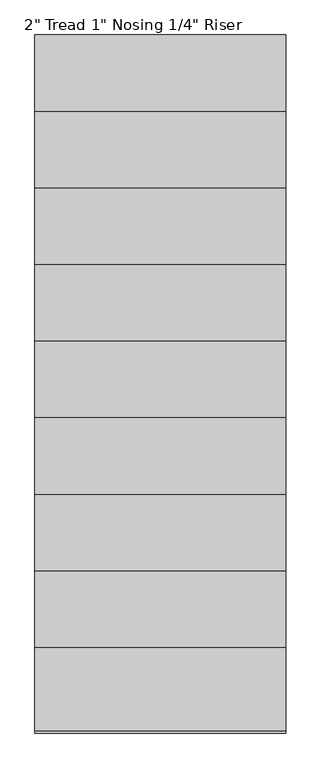
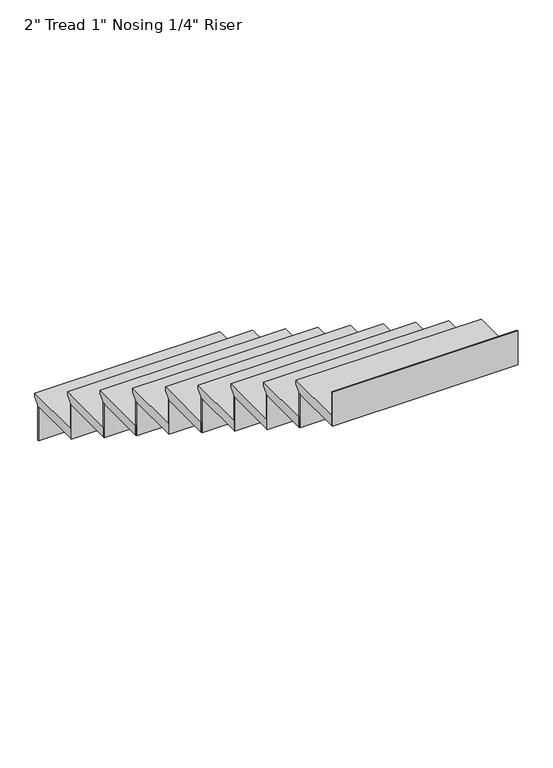
"""IFC4 building model written with IfcOpenShell, lengths in millimetres: stair flight geometry."""

from ifc_helpers import new_model, si_unit, frame, origin, place, context, project, spatial, polyline, outline, extrude, source, transform, mapped, element, save


def stair_flight_364c9dde(model_context):
    return source(origin(), model_context, "Body", "SweptSolid", [
        extrude(outline(polyline([(1808.6257925, 8610.6), (2113.4257925, 8610.6), (2113.4257925, 8591.55), (2088.0257925, 8566.15), (2088.0257925, 8559.8), (1808.6257925, 8559.8), (1808.6257925, 8610.6)])), frame((1465.4501403, 0.0, 0.0), z_axis=(1.0, 0.0, 0.0), x_axis=(0.0, 1.0, 0.0)), (0.0, 0.0, 1.0), 914.4),
        extrude(outline(polyline([(1465.4501403, 2081.6757925), (1465.4501403, 2088.0257925), (2379.8501403, 2088.0257925), (2379.8501403, 2081.6757925), (1465.4501403, 2081.6757925)])), frame((0.0, 0.0, 8382.0), z_axis=(0.0, 0.0, 1.0), x_axis=(1.0, 0.0, 0.0)), (0.0, 0.0, 1.0), 177.8),
        extrude(outline(polyline([(1465.4501403, 1802.2757925), (1465.4501403, 1808.6257925), (2379.8501403, 1808.6257925), (2379.8501403, 1802.2757925), (1465.4501403, 1802.2757925)])), frame((0.0, 0.0, 8559.8), z_axis=(0.0, 0.0, 1.0), x_axis=(1.0, 0.0, 0.0)), (0.0, 0.0, 1.0), 177.8),
        extrude(outline(polyline([(1529.2257925, 8788.4), (1834.0257925, 8788.4), (1834.0257925, 8769.35), (1808.6257925, 8743.95), (1808.6257925, 8737.6), (1529.2257925, 8737.6), (1529.2257925, 8788.4)])), frame((1465.4501403, 0.0, 0.0), z_axis=(1.0, 0.0, 0.0), x_axis=(0.0, 1.0, 0.0)), (0.0, 0.0, 1.0), 914.4),
        extrude(outline(polyline([(1465.4501403, 1522.8757925), (1465.4501403, 1529.2257925), (2379.8501403, 1529.2257925), (2379.8501403, 1522.8757925), (1465.4501403, 1522.8757925)])), frame((0.0, 0.0, 8737.6), z_axis=(0.0, 0.0, 1.0), x_axis=(1.0, 0.0, 0.0)), (0.0, 0.0, 1.0), 177.8),
        extrude(outline(polyline([(1249.8257925, 8966.2), (1554.6257925, 8966.2), (1554.6257925, 8947.15), (1529.2257925, 8921.75), (1529.2257925, 8915.4), (1249.8257925, 8915.4), (1249.8257925, 8966.2)])), frame((1465.4501403, 0.0, 0.0), z_axis=(1.0, 0.0, 0.0), x_axis=(0.0, 1.0, 0.0)), (0.0, 0.0, 1.0), 914.4),
        extrude(outline(polyline([(1465.4501403, 1243.4757925), (1465.4501403, 1249.8257925), (2379.8501403, 1249.8257925), (2379.8501403, 1243.4757925), (1465.4501403, 1243.4757925)])), frame((0.0, 0.0, 8915.4), z_axis=(0.0, 0.0, 1.0), x_axis=(1.0, 0.0, 0.0)), (0.0, 0.0, 1.0), 177.8),
        extrude(outline(polyline([(970.4257925, 9144.0), (1275.2257925, 9144.0), (1275.2257925, 9124.95), (1249.8257925, 9099.55), (1249.8257925, 9093.2), (970.4257925, 9093.2), (970.4257925, 9144.0)])), frame((1465.4501403, 0.0, 0.0), z_axis=(1.0, 0.0, 0.0), x_axis=(0.0, 1.0, 0.0)), (0.0, 0.0, 1.0), 914.4),
        extrude(outline(polyline([(1465.4501403, 964.0757925), (1465.4501403, 970.4257925), (2379.8501403, 970.4257925), (2379.8501403, 964.0757925), (1465.4501403, 964.0757925)])), frame((0.0, 0.0, 9093.2), z_axis=(0.0, 0.0, 1.0), x_axis=(1.0, 0.0, 0.0)), (0.0, 0.0, 1.0), 177.8),
        extrude(outline(polyline([(691.0257925, 9321.8), (995.8257925, 9321.8), (995.8257925, 9302.75), (970.4257925, 9277.35), (970.4257925, 9271.0), (691.0257925, 9271.0), (691.0257925, 9321.8)])), frame((1465.4501403, 0.0, 0.0), z_axis=(1.0, 0.0, 0.0), x_axis=(0.0, 1.0, 0.0)), (0.0, 0.0, 1.0), 914.4),
        extrude(outline(polyline([(1465.4501403, 684.6757925), (1465.4501403, 691.0257925), (2379.8501403, 691.0257925), (2379.8501403, 684.6757925), (1465.4501403, 684.6757925)])), frame((0.0, 0.0, 9271.0), z_axis=(0.0, 0.0, 1.0), x_axis=(1.0, 0.0, 0.0)), (0.0, 0.0, 1.0), 177.8),
        extrude(outline(polyline([(411.6257925, 9499.6), (716.4257925, 9499.6), (716.4257925, 9480.55), (691.0257925, 9455.15), (691.0257925, 9448.8), (411.6257925, 9448.8), (411.6257925, 9499.6)])), frame((1465.4501403, 0.0, 0.0), z_axis=(1.0, 0.0, 0.0), x_axis=(0.0, 1.0, 0.0)), (0.0, 0.0, 1.0), 914.4),
        extrude(outline(polyline([(1465.4501403, 405.2757925), (1465.4501403, 411.6257925), (2379.8501403, 411.6257925), (2379.8501403, 405.2757925), (1465.4501403, 405.2757925)])), frame((0.0, 0.0, 9448.8), z_axis=(0.0, 0.0, 1.0), x_axis=(1.0, 0.0, 0.0)), (0.0, 0.0, 1.0), 177.8),
        extrude(outline(polyline([(132.2257925, 9677.4), (437.0257925, 9677.4), (437.0257925, 9658.35), (411.6257925, 9632.95), (411.6257925, 9626.6), (132.2257925, 9626.6), (132.2257925, 9677.4)])), frame((1465.4501403, 0.0, 0.0), z_axis=(1.0, 0.0, 0.0), x_axis=(0.0, 1.0, 0.0)), (0.0, 0.0, 1.0), 914.4),
        extrude(outline(polyline([(1465.4501403, 125.8757925), (1465.4501403, 132.2257925), (2379.8501403, 132.2257925), (2379.8501403, 125.8757925), (1465.4501403, 125.8757925)])), frame((0.0, 0.0, 9626.6), z_axis=(0.0, 0.0, 1.0), x_axis=(1.0, 0.0, 0.0)), (0.0, 0.0, 1.0), 177.8),
        extrude(outline(polyline([(-147.1742075, 9855.2), (157.6257925, 9855.2), (157.6257925, 9836.15), (132.2257925, 9810.75), (132.2257925, 9804.4), (-147.1742075, 9804.4), (-147.1742075, 9855.2)])), frame((1465.4501403, 0.0, 0.0), z_axis=(1.0, 0.0, 0.0), x_axis=(0.0, 1.0, 0.0)), (0.0, 0.0, 1.0), 914.4),
        extrude(outline(polyline([(1465.4501403, -153.5242075), (1465.4501403, -147.1742075), (2379.8501403, -147.1742075), (2379.8501403, -153.5242075), (1465.4501403, -153.5242075)])), frame((0.0, 0.0, 9804.4), z_axis=(0.0, 0.0, 1.0), x_axis=(1.0, 0.0, 0.0)), (0.0, 0.0, 1.0), 177.8),
        extrude(outline(polyline([(1465.4501403, -432.9242075), (1465.4501403, -426.5742075), (2379.8501403, -426.5742075), (2379.8501403, -432.9242075), (1465.4501403, -432.9242075)])), frame((0.0, 0.0, 9982.2), z_axis=(0.0, 0.0, 1.0), x_axis=(1.0, 0.0, 0.0)), (0.0, 0.0, 1.0), 177.8),
        extrude(outline(polyline([(-426.5742075, 10033.0), (-121.7742075, 10033.0), (-121.7742075, 10013.95), (-147.1742075, 9988.55), (-147.1742075, 9982.2), (-426.5742075, 9982.2), (-426.5742075, 10033.0)])), frame((1465.4501403, 0.0, 0.0), z_axis=(1.0, 0.0, 0.0), x_axis=(0.0, 1.0, 0.0)), (0.0, 0.0, 1.0), 914.4),
    ])


if __name__ == "__main__":
    model = new_model("IFC4")
    model_context = context("Model", 3, world=origin())
    ifc_project = project(units=[si_unit("LENGTHUNIT", "METRE", prefix="MILLI")], contexts=[model_context])
    site = spatial("IfcSite", under=ifc_project)
    building = spatial("IfcBuilding", under=site)
    placement = place(None, origin())
    stair_flight_shape = stair_flight_364c9dde(model_context)
    element("IfcStairFlight", 1, ObjectType="2\" Tread 1\" Nosing 1/4\" Riser", at=placement, inside=building, context=model_context, shape_type="MappedRepresentation", body=[
        mapped(stair_flight_shape, transform((0.0, 0.0, 0.0), x_axis=(1.0, 0.0, 0.0), y_axis=(0.0, 1.0, 0.0), z_axis=(0.0, 0.0, 1.0))),
    ])
    save(model, "model.ifc")
